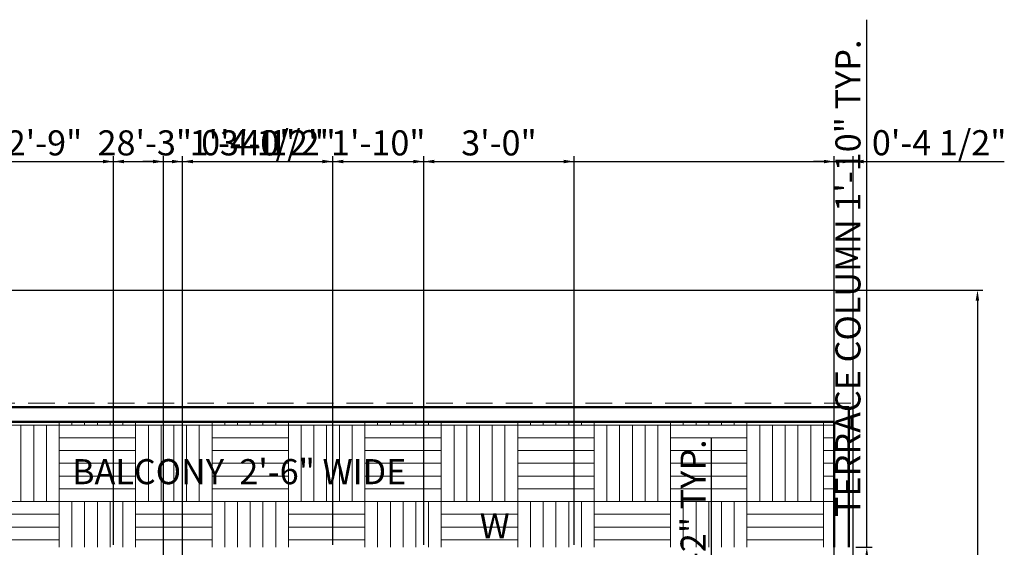
# Model space of a CAD drawing. Units: millimetres. Extents: x 67033 to 68301, y 155969 to 157209.
# Tile 16 of 17: x 67638 to 67873, y 157083 to 157209. Entities that reach past the tile are written whole.
import ezdxf

# ---------------------------------------------------------------- set-up
doc = ezdxf.new("R2010")
doc.units = ezdxf.units.MM
doc.linetypes.add('HIDDEN', pattern=[9.525, 6.35, -3.175])
for name, color, linetype, lineweight in [('A-ANNO-DIMS', 2, 'Continuous', 18), ('A-ANNO-TEXT', 7, 'Continuous', 18), ('A-AREA-IDEN', 3, 'Continuous', 18), ('A-FLOR-OVHD', 1, 'HIDDEN', 18), ('A-FLOR-PATT', 252, 'Continuous', 13), ('A-WALL', 7, 'Continuous', 50)]:
    doc.layers.add(name, color=color, linetype=linetype, lineweight=lineweight)
doc.styles.get("Standard").update_dxf_attribs({"font": 'arial.ttf'})
doc.dimstyles.new('ISO-25', dxfattribs={"dimtxt": 6, "dimasz": 2.5, "dimexe": 1.25, "dimexo": 0.625, "dimtad": 1, "dimdec": 0, "dimlunit": 3, "dimtxsty": 'Standard', "dimcen": 2.5, "dimadec": 0, "dimazin": 0, "dimtfac": 1, "dimtdec": 0, "dimtmove": 0, "dimatfit": 3, "dimfxl": 1, "dimarcsym": 0})

# ---------------------------------------------------------------- blocks, each defined once
blk = doc.blocks.new('*D64')
at = {"layer": 'A-ANNO-DIMS', "color": 0, "lineweight": -2, "transparency": 16777216}
for p, q in [((67803.43, 157069.35), (67803.43, 157109.11)), ((67800.69, 157069.35), (67804.68, 157069.35)), ((67803.43, 157057.6), (67803.43, 157066.85)), ((67800.69, 157055.1), (67804.68, 157055.1))]:
    blk.add_line(p, q, dxfattribs=at)
at = {"layer": 'A-ANNO-DIMS', "color": 0, "transparency": 16777216}
for points in [[(67803.01, 157066.85), (67803.85, 157066.85), (67803.43, 157069.35)], [(67803.01, 157057.6), (67803.85, 157057.6), (67803.43, 157055.1)]]:
    blk.add_solid(points, dxfattribs=at)
at = {"layer": 'Defpoints', "color": 0, "transparency": 16777216}
for p in [(67800.07, 157069.35), (67803.43, 157069.35), (67800.07, 157055.1)]:
    blk.add_point(p, dxfattribs=at)
at = {"layer": 'A-ANNO-DIMS', "color": 0, "transparency": 16777216, "insert": (67799.79, 157090.48), "char_height": 6, "attachment_point": 5, "rotation": 90}
blk.add_mtext('1\'-2" TYP.', dxfattribs=at)
blk = doc.blocks.new('*D69')
at = {"layer": 'A-ANNO-DIMS', "color": 0, "lineweight": -2, "transparency": 16777216}
for p, q in [((67840.59, 157082.99), (67840.59, 157209.16)), ((67837.94, 157082.99), (67841.84, 157082.99)), ((67840.59, 157063.69), (67840.59, 157080.49)), ((67837.94, 157061.19), (67841.84, 157061.19))]:
    blk.add_line(p, q, dxfattribs=at)
at = {"layer": 'A-ANNO-DIMS', "color": 0, "transparency": 16777216}
for points in [[(67840.17, 157080.49), (67841, 157080.49), (67840.59, 157082.99)], [(67840.17, 157063.69), (67841, 157063.69), (67840.59, 157061.19)]]:
    blk.add_solid(points, dxfattribs=at)
at = {"layer": 'Defpoints', "color": 0, "transparency": 16777216}
for p in [(67837.32, 157082.99), (67840.59, 157082.99), (67837.32, 157061.19)]:
    blk.add_point(p, dxfattribs=at)
at = {"layer": 'A-ANNO-DIMS', "color": 0, "transparency": 16777216, "insert": (67836.86, 157147.33), "char_height": 6, "attachment_point": 5, "rotation": 90}
blk.add_mtext('TERRACE COLUMN 1\'-10" TYP.', dxfattribs=at)
blk = doc.blocks.new('*D98')
at = {"layer": 'A-ANNO-DIMS', "color": 0, "lineweight": -2, "transparency": 16777216}
for p, q in [((67627.32, 157083.62), (67627.32, 157176.49)), ((67660.32, 157083.62), (67660.32, 157176.49)), ((67629.82, 157175.24), (67657.82, 157175.24))]:
    blk.add_line(p, q, dxfattribs=at)
at = {"layer": 'A-ANNO-DIMS', "color": 0, "transparency": 16777216}
for points in [[(67629.82, 157175.66), (67629.82, 157174.83), (67627.32, 157175.24)], [(67657.82, 157175.66), (67657.82, 157174.83), (67660.32, 157175.24)]]:
    blk.add_solid(points, dxfattribs=at)
at = {"layer": 'Defpoints', "color": 0, "transparency": 16777216}
for p in [(67660.32, 157175.24), (67627.32, 157082.99), (67660.32, 157082.99)]:
    blk.add_point(p, dxfattribs=at)
at = {"layer": 'A-ANNO-DIMS', "color": 0, "transparency": 16777216, "insert": (67643.82, 157178.93), "char_height": 6, "attachment_point": 5}
blk.add_mtext('2\'-9"', dxfattribs=at)
blk = doc.blocks.new('*D99')
at = {"layer": 'A-ANNO-DIMS', "color": 0, "lineweight": -2, "transparency": 16777216}
for p, q in [((67660.32, 157083.62), (67660.32, 157176.49)), ((67676.82, 157083.62), (67676.82, 157176.49)), ((67662.82, 157175.24), (67674.32, 157175.24)), ((67676.82, 157175.24), (67709.93, 157175.24))]:
    blk.add_line(p, q, dxfattribs=at)
at = {"layer": 'A-ANNO-DIMS', "color": 0, "transparency": 16777216}
for points in [[(67662.82, 157175.66), (67662.82, 157174.83), (67660.32, 157175.24)], [(67674.32, 157175.66), (67674.32, 157174.83), (67676.82, 157175.24)]]:
    blk.add_solid(points, dxfattribs=at)
at = {"layer": 'Defpoints', "color": 0, "transparency": 16777216}
for p in [(67676.82, 157175.24), (67660.32, 157082.99), (67676.82, 157082.99)]:
    blk.add_point(p, dxfattribs=at)
at = {"layer": 'A-ANNO-DIMS', "color": 0, "transparency": 16777216, "insert": (67694.62, 157178.97), "char_height": 6, "attachment_point": 5}
blk.add_mtext('1\'-4 1/2"', dxfattribs=at)
blk = doc.blocks.new('*D100')
at = {"layer": 'A-ANNO-DIMS', "color": 0, "lineweight": -2, "transparency": 16777216}
for p, q in [((67676.82, 157083.62), (67676.82, 157176.49)), ((67712.82, 157083.62), (67712.82, 157176.49)), ((67679.32, 157175.24), (67710.32, 157175.24))]:
    blk.add_line(p, q, dxfattribs=at)
at = {"layer": 'A-ANNO-DIMS', "color": 0, "transparency": 16777216}
for points in [[(67679.32, 157175.66), (67679.32, 157174.83), (67676.82, 157175.24)], [(67710.32, 157175.66), (67710.32, 157174.83), (67712.82, 157175.24)]]:
    blk.add_solid(points, dxfattribs=at)
at = {"layer": 'Defpoints', "color": 0, "transparency": 16777216}
for p in [(67712.82, 157175.24), (67676.82, 157082.99), (67712.82, 157082.99)]:
    blk.add_point(p, dxfattribs=at)
at = {"layer": 'A-ANNO-DIMS', "color": 0, "transparency": 16777216, "insert": (67694.82, 157178.93), "char_height": 6, "attachment_point": 5}
blk.add_mtext('3\'-0"', dxfattribs=at)
blk = doc.blocks.new('*D101')
at = {"layer": 'A-ANNO-DIMS', "color": 0, "lineweight": -2, "transparency": 16777216}
for p, q in [((67712.82, 157083.62), (67712.82, 157176.49)), ((67734.57, 157083.62), (67734.57, 157176.49)), ((67715.32, 157175.24), (67732.07, 157175.24))]:
    blk.add_line(p, q, dxfattribs=at)
at = {"layer": 'A-ANNO-DIMS', "color": 0, "transparency": 16777216}
for points in [[(67715.32, 157175.66), (67715.32, 157174.83), (67712.82, 157175.24)], [(67732.07, 157175.66), (67732.07, 157174.83), (67734.57, 157175.24)]]:
    blk.add_solid(points, dxfattribs=at)
at = {"layer": 'Defpoints', "color": 0, "transparency": 16777216}
for p in [(67734.57, 157175.24), (67712.82, 157082.99), (67734.57, 157082.99)]:
    blk.add_point(p, dxfattribs=at)
at = {"layer": 'A-ANNO-DIMS', "color": 0, "transparency": 16777216, "insert": (67723.69, 157178.93), "char_height": 6, "attachment_point": 5}
blk.add_mtext('1\'-10"', dxfattribs=at)
blk = doc.blocks.new('*D102')
at = {"layer": 'A-ANNO-DIMS', "color": 0, "lineweight": -2, "transparency": 16777216}
for p, q in [((67734.57, 157083.62), (67734.57, 157176.49)), ((67770.57, 157083.62), (67770.57, 157176.49)), ((67737.07, 157175.24), (67768.07, 157175.24))]:
    blk.add_line(p, q, dxfattribs=at)
at = {"layer": 'A-ANNO-DIMS', "color": 0, "transparency": 16777216}
for points in [[(67737.07, 157175.66), (67737.07, 157174.83), (67734.57, 157175.24)], [(67768.07, 157175.66), (67768.07, 157174.83), (67770.57, 157175.24)]]:
    blk.add_solid(points, dxfattribs=at)
at = {"layer": 'Defpoints', "color": 0, "transparency": 16777216}
for p in [(67770.57, 157175.24), (67734.57, 157082.99), (67770.57, 157082.99)]:
    blk.add_point(p, dxfattribs=at)
at = {"layer": 'A-ANNO-DIMS', "color": 0, "transparency": 16777216, "insert": (67752.57, 157178.93), "char_height": 6, "attachment_point": 5}
blk.add_mtext('3\'-0"', dxfattribs=at)
blk = doc.blocks.new('*D111')
at = {"layer": 'A-ANNO-DIMS', "color": 0, "lineweight": -2, "transparency": 16777216}
for p, q in [((67498.32, 157137.62), (67498.32, 157176.49)), ((67837.32, 157083.62), (67837.32, 157176.49)), ((67500.82, 157175.24), (67834.82, 157175.24))]:
    blk.add_line(p, q, dxfattribs=at)
at = {"layer": 'A-ANNO-DIMS', "color": 0, "transparency": 16777216}
for points in [[(67500.82, 157175.66), (67500.82, 157174.83), (67498.32, 157175.24)], [(67834.82, 157175.66), (67834.82, 157174.83), (67837.32, 157175.24)]]:
    blk.add_solid(points, dxfattribs=at)
at = {"layer": 'Defpoints', "color": 0, "transparency": 16777216}
for p in [(67837.32, 157175.24), (67498.32, 157136.99), (67837.32, 157082.99)]:
    blk.add_point(p, dxfattribs=at)
at = {"layer": 'A-ANNO-DIMS', "color": 0, "transparency": 16777216, "insert": (67667.82, 157178.93), "char_height": 6, "attachment_point": 5}
blk.add_mtext('28\'-3"', dxfattribs=at)
blk = doc.blocks.new('*D112')
at = {"layer": 'A-ANNO-DIMS', "color": 0, "lineweight": -2, "transparency": 16777216}
for p, q in [((67601.44, 157144.49), (67868.32, 157144.49)), ((67867.07, 157141.99), (67867.07, 156564.99)), ((67768.94, 156562.49), (67868.32, 156562.49))]:
    blk.add_line(p, q, dxfattribs=at)
at = {"layer": 'A-ANNO-DIMS', "color": 0, "transparency": 16777216}
for points in [[(67866.65, 157141.99), (67867.48, 157141.99), (67867.07, 157144.49)], [(67866.65, 156564.99), (67867.48, 156564.99), (67867.07, 156562.49)]]:
    blk.add_solid(points, dxfattribs=at)
at = {"layer": 'Defpoints', "color": 0, "transparency": 16777216}
for p in [(67600.82, 157144.49), (67768.32, 156562.49), (67867.07, 156562.49)]:
    blk.add_point(p, dxfattribs=at)
at = {"layer": 'A-ANNO-DIMS', "color": 0, "transparency": 16777216, "insert": (67863.38, 156853.49), "char_height": 6, "attachment_point": 5, "rotation": 90}
blk.add_mtext('48\'-6"', dxfattribs=at)
blk = doc.blocks.new('*D115')
at = {"layer": 'A-ANNO-DIMS', "color": 0, "lineweight": -2, "transparency": 16777216}
for p, q in [((67672.32, 156960.62), (67672.32, 157176.49)), ((67676.82, 156960.62), (67676.82, 157176.49)), ((67669.82, 157175.24), (67667.32, 157175.24)), ((67672.32, 157175.24), (67676.82, 157175.24)), ((67679.32, 157175.24), (67713, 157175.24))]:
    blk.add_line(p, q, dxfattribs=at)
at = {"layer": 'A-ANNO-DIMS', "color": 0, "transparency": 16777216}
for points in [[(67669.82, 157175.66), (67669.82, 157174.83), (67672.32, 157175.24)], [(67679.32, 157175.66), (67679.32, 157174.83), (67676.82, 157175.24)]]:
    blk.add_solid(points, dxfattribs=at)
at = {"layer": 'Defpoints', "color": 0, "transparency": 16777216}
for p in [(67676.82, 157175.24), (67672.32, 156959.99), (67676.82, 156959.99)]:
    blk.add_point(p, dxfattribs=at)
at = {"layer": 'A-ANNO-DIMS', "color": 0, "transparency": 16777216, "insert": (67697.41, 157178.97), "char_height": 6, "attachment_point": 5}
blk.add_mtext('0\'-4 1/2"', dxfattribs=at)
blk = doc.blocks.new('*D116')
at = {"layer": 'A-ANNO-DIMS', "color": 0, "lineweight": -2, "transparency": 16777216}
for p, q in [((67832.82, 157061.82), (67832.82, 157176.49)), ((67837.32, 157061.82), (67837.32, 157176.49)), ((67830.32, 157175.24), (67827.82, 157175.24)), ((67832.82, 157175.24), (67837.32, 157175.24)), ((67839.82, 157175.24), (67873.5, 157175.24))]:
    blk.add_line(p, q, dxfattribs=at)
at = {"layer": 'A-ANNO-DIMS', "color": 0, "transparency": 16777216}
for points in [[(67830.32, 157175.66), (67830.32, 157174.83), (67832.82, 157175.24)], [(67839.82, 157175.66), (67839.82, 157174.83), (67837.32, 157175.24)]]:
    blk.add_solid(points, dxfattribs=at)
at = {"layer": 'Defpoints', "color": 0, "transparency": 16777216}
for p in [(67837.32, 157175.24), (67832.82, 157061.19), (67837.32, 157061.19)]:
    blk.add_point(p, dxfattribs=at)
at = {"layer": 'A-ANNO-DIMS', "color": 0, "transparency": 16777216, "insert": (67857.91, 157178.97), "char_height": 6, "attachment_point": 5}
blk.add_mtext('0\'-4 1/2"', dxfattribs=at)

msp = doc.modelspace()

# ---------------------------------------------------------------- hatches: boundary and pattern name
at = {"layer": 'A-FLOR-PATT'}
h = msp.add_hatch(dxfattribs=at)
h.set_pattern_fill('AR-PARQ1', color=256, scale=0.06)
h.paths.add_polyline_path([(67832.82, 157112.99), (67597.32, 157112.99), (67597.32, 157140.99), (67567.32, 157140.99), (67567.32, 157082.99), (67627.32, 157082.99), (67660.32, 157082.99), (67832.82, 157082.99)])
h.paths.add_polyline_path([(67595.94, 157081.09), (67613.84, 157081.09), (67613.84, 157093.46), (67595.94, 157093.46)], flags=9)
h.paths.add_polyline_path([(67740.95, 157081.83), (67758.84, 157081.83), (67758.84, 157094.2), (67740.95, 157094.2)], flags=9)

# ---------------------------------------------------------------- linework, layer by layer
at = {"layer": 'A-FLOR-OVHD'}
for p in [(67601.82, 157117.49), (67837.32, 157082.99)]:
    msp.add_line(p, (67837.32, 157117.49), dxfattribs=at)
at = {"layer": 'A-WALL'}
for p, q in [((67600.82, 157116.49), (67836.32, 157116.49)), ((67836.32, 157116.49), (67836.32, 157082.99)), ((67597.32, 157112.99), (67832.82, 157112.99)), ((67832.82, 157112.99), (67832.82, 157082.99))]:
    msp.add_line(p, q, dxfattribs=at)

# ---------------------------------------------------------------- texts
at = {"layer": 'A-ANNO-TEXT', "insert": (67742.45, 157091.11), "char_height": 6, "attachment_point": 1}
msp.add_mtext_dynamic_manual_height_columns('   W', width=19.5287, gutter_width=12.5, heights=[0], dxfattribs=at)
at = {"layer": 'A-AREA-IDEN', "insert": (67648.58, 157104.08), "char_height": 6, "attachment_point": 1}
msp.add_mtext_dynamic_manual_height_columns(' BALCONY  2\'-6" WIDE', width=93.5859, gutter_width=12.5, heights=[0], dxfattribs=at)

# ---------------------------------------------------------------- dimensions: what is measured, and where the dimension line sits
at = {"layer": 'A-ANNO-DIMS'}
for base, p1, p2, text, picture, middle in [((67840.59, 157082.99), (67837.32, 157061.19), (67837.32, 157082.99), 'TERRACE COLUMN <> TYP.', '*D69', (67836.86, 157147.33)), ((67803.431, 157069.3533), (67800.0652, 157055.1037), (67800.0652, 157069.3533), '<> TYP.', '*D64', (67799.7916, 157090.4824))]:
    dim = msp.add_linear_dim(base=base, p1=p1, p2=p2, angle=90, text=text, dimstyle='ISO-25', override={"dimdec": 1, "dimrnd": 0, "dimzin": 1, "dimlunit": 4, "dimfrac": 2}, dxfattribs=at)
    dim.commit()
    dim.dimension.update_dxf_attribs({"geometry": picture, "text_midpoint": middle})
for base, p1, p2, picture, middle in [((67676.82, 157175.24), (67660.32, 157082.99), (67676.82, 157082.99), '*D99', (67694.62, 157178.97)), ((67676.82, 157175.24), (67672.32, 156959.99), (67676.82, 156959.99), '*D115', (67697.41, 157178.97)), ((67837.32, 157175.24), (67832.82, 157061.19), (67837.32, 157061.19), '*D116', (67857.91, 157178.97)), ((67837.32, 157175.24), (67498.32, 157136.99), (67837.32, 157082.99), '*D111', (67667.82, 157178.93)), ((67660.32, 157175.24), (67627.32, 157082.99), (67660.32, 157082.99), '*D98', (67643.82, 157178.93)), ((67712.82, 157175.24), (67676.82, 157082.99), (67712.82, 157082.99), '*D100', (67694.82, 157178.93)), ((67734.565057, 157175.244117), (67712.815057, 157082.994117), (67734.565057, 157082.994117), '*D101', (67723.690057, 157178.93255493)), ((67770.57, 157175.24), (67734.57, 157082.99), (67770.57, 157082.99), '*D102', (67752.57, 157178.93))]:
    dim = msp.add_linear_dim(base=base, p1=p1, p2=p2, dimstyle='ISO-25', override={"dimdec": 1, "dimlfac": 1, "dimrnd": 0, "dimzin": 1, "dimdsep": 46, "dimlunit": 4, "dimfrac": 2}, dxfattribs=at)
    dim.commit()
    dim.dimension.update_dxf_attribs({"geometry": picture, "text_midpoint": middle})
dim = msp.add_linear_dim(base=(67867.07, 156562.49), p1=(67600.82, 157144.49), p2=(67768.32, 156562.49), angle=90, dimstyle='ISO-25', override={"dimdec": 1, "dimlfac": 1, "dimrnd": 0, "dimzin": 1, "dimdsep": 46, "dimlunit": 4, "dimfrac": 2}, dxfattribs=at)
dim.commit()
dim.dimension.update_dxf_attribs({"geometry": '*D112', "text_midpoint": (67863.38, 156853.49)})

doc.saveas('drawing.dxf')
